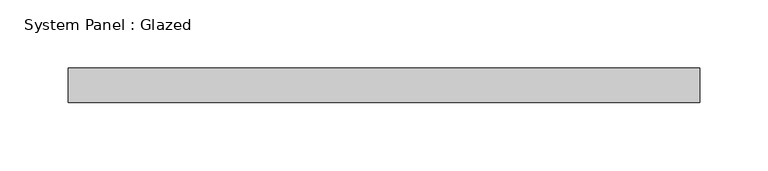
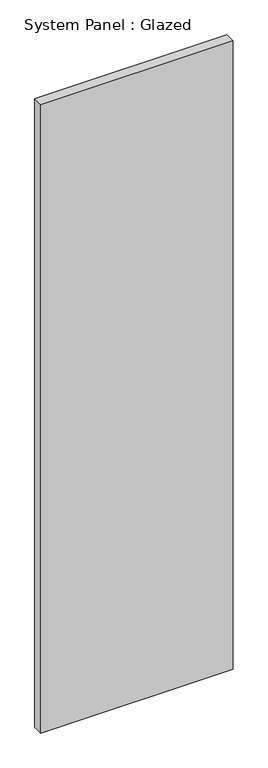
"""IFC4 building model written with IfcOpenShell, lengths in millimetres: plate geometry, System Panel : Glazed."""

from ifc_helpers import new_model, si_unit, origin, origin_with_axes, place, context, project, spatial, polyline, outline, extrude, source, transform, mapped, element, save


def system_panel_glazed_096f46ea(model_context):
    return source(origin(), model_context, "Body", "SweptSolid", [
        extrude(outline(polyline([(231.775, 19.05), (-231.775, 19.05), (-231.775, 44.45), (231.775, 44.45), (231.775, 19.05)])), origin_with_axes(), (0.0, 0.0, 1.0), 1601.1374524),
    ])


if __name__ == "__main__":
    model = new_model("IFC4")
    model_context = context("Model", 3, world=origin())
    ifc_project = project(units=[si_unit("LENGTHUNIT", "METRE", prefix="MILLI")], contexts=[model_context])
    site = spatial("IfcSite", under=ifc_project)
    building = spatial("IfcBuilding", under=site)
    placement = place(None, origin())
    system_panel_glazed_shape = system_panel_glazed_096f46ea(model_context)
    element("IfcPlate", 1, ObjectType="System Panel : Glazed", at=placement, inside=building, context=model_context, shape_type="MappedRepresentation", body=[
        mapped(system_panel_glazed_shape, transform((0.0, 0.0, 0.0), x_axis=(1.0, 0.0, 0.0), y_axis=(0.0, 1.0, 0.0), z_axis=(0.0, 0.0, 1.0))),
    ])
    save(model, "model.ifc")

# Revit data of these elements
# Type "System Panel : Glazed"
#   Construction Type Id = "GSP4R"
#   Analytic Construction = "1/8 in Pilkington single glazing"
#   Visual Light Transmittance = 0.9
#   Solar Heat Gain Coefficient = 0.86
#   Heat Transfer Coefficient (U) = 1.18115 BTU/(h·ft²·°F)
#   Define Thermal Properties by = 1
# Element 1 (IfcPlate, "System Panel : Glazed")
#   Materials on its faces: "Glass"
# Materials
#   "Glass": class "Glass", colour RGB 0 128 192, transparency 0.75, Description = "Soda Lime Glass", Cost = 0
